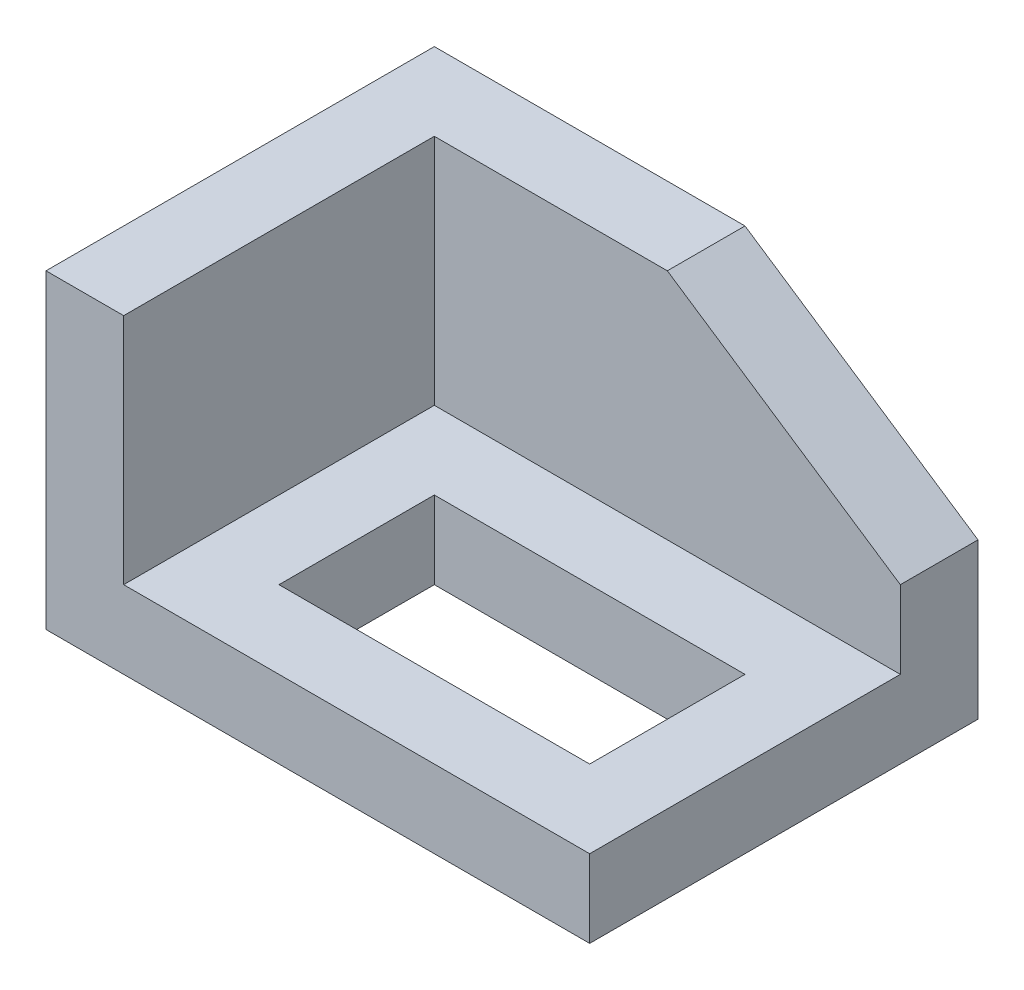
ISO-10303-21;
HEADER;
FILE_DESCRIPTION(('STEP AP214'),'2;1');
FILE_NAME('part.step','',(''),(''),'','','');
FILE_SCHEMA(('AUTOMOTIVE_DESIGN { 1 0 10303 214 1 1 1 1 }'));
ENDSEC;
DATA;
#1=APPLICATION_CONTEXT('core data for automotive mechanical design processes');
#2=APPLICATION_PROTOCOL_DEFINITION('international standard','automotive_design',2000,#1);
#3=PRODUCT_CONTEXT('',#1,'mechanical');
#4=PRODUCT('Part','Part','',(#3));
#5=PRODUCT_RELATED_PRODUCT_CATEGORY('part','',(#4));
#6=PRODUCT_DEFINITION_FORMATION('','',#4);
#7=PRODUCT_DEFINITION_CONTEXT('part definition',#1,'design');
#8=PRODUCT_DEFINITION('design','',#6,#7);
#9=PRODUCT_DEFINITION_SHAPE('','',#8);
#10=(LENGTH_UNIT() NAMED_UNIT(*) SI_UNIT(.MILLI.,.METRE.));
#11=(NAMED_UNIT(*) PLANE_ANGLE_UNIT() SI_UNIT($,.RADIAN.));
#12=(NAMED_UNIT(*) SI_UNIT($,.STERADIAN.) SOLID_ANGLE_UNIT());
#13=UNCERTAINTY_MEASURE_WITH_UNIT(LENGTH_MEASURE(1.E-05),#10,'distance_accuracy_value','');
#14=(GEOMETRIC_REPRESENTATION_CONTEXT(3) GLOBAL_UNCERTAINTY_ASSIGNED_CONTEXT((#13)) GLOBAL_UNIT_ASSIGNED_CONTEXT((#10,
#11,#12)) REPRESENTATION_CONTEXT('',''));
#15=CARTESIAN_POINT('',(0.,0.,0.));
#16=DIRECTION('',(0.,0.,1.));
#17=DIRECTION('',(1.,0.,0.));
#18=AXIS2_PLACEMENT_3D('',#15,#16,#17);
#19=CARTESIAN_POINT('',(0.,0.,10.));
#20=DIRECTION('',(0.,0.,1.));
#21=DIRECTION('',(1.,0.,0.));
#22=AXIS2_PLACEMENT_3D('',#19,#20,#21);
#23=PLANE('',#22);
#24=DIRECTION('',(0.,1.,0.));
#25=VECTOR('',#24,1.);
#26=CARTESIAN_POINT('',(10.,40.,10.));
#27=LINE('',#26,#25);
#28=CARTESIAN_POINT('',(10.,10.,10.));
#29=VERTEX_POINT('',#28);
#30=CARTESIAN_POINT('',(10.,40.,10.));
#31=VERTEX_POINT('',#30);
#32=EDGE_CURVE('E182',#29,#31,#27,.T.);
#33=ORIENTED_EDGE('',*,*,#32,.F.);
#34=DIRECTION('',(-1.,0.,0.));
#35=VECTOR('',#34,1.);
#36=CARTESIAN_POINT('',(10.,10.,10.));
#37=LINE('',#36,#35);
#38=CARTESIAN_POINT('',(70.,10.,10.));
#39=VERTEX_POINT('',#38);
#40=EDGE_CURVE('E167',#39,#29,#37,.T.);
#41=ORIENTED_EDGE('',*,*,#40,.F.);
#42=DIRECTION('',(0.,1.,0.));
#43=VECTOR('',#42,1.);
#44=CARTESIAN_POINT('',(70.,0.,10.));
#45=LINE('',#44,#43);
#46=CARTESIAN_POINT('',(70.,20.,10.));
#47=VERTEX_POINT('',#46);
#48=EDGE_CURVE('E196',#39,#47,#45,.T.);
#49=ORIENTED_EDGE('',*,*,#48,.T.);
#50=DIRECTION('',(-0.832050294337844,0.554700196225229,0.));
#51=VECTOR('',#50,1.);
#52=CARTESIAN_POINT('',(70.,20.,10.));
#53=LINE('',#52,#51);
#54=CARTESIAN_POINT('',(40.,40.,10.));
#55=VERTEX_POINT('',#54);
#56=EDGE_CURVE('E199',#47,#55,#53,.T.);
#57=ORIENTED_EDGE('',*,*,#56,.T.);
#58=DIRECTION('',(-1.,0.,0.));
#59=VECTOR('',#58,1.);
#60=CARTESIAN_POINT('',(0.,40.,10.));
#61=LINE('',#60,#59);
#62=EDGE_CURVE('E201',#55,#31,#61,.T.);
#63=ORIENTED_EDGE('',*,*,#62,.T.);
#64=EDGE_LOOP('',(#33,#41,#49,#57,#63));
#65=FACE_BOUND('',#64,.T.);
#66=ADVANCED_FACE('F44',(#65),#23,.T.);
#67=CARTESIAN_POINT('',(10.,40.,50.));
#68=DIRECTION('',(-1.,0.,0.));
#69=DIRECTION('',(0.,-1.,0.));
#70=AXIS2_PLACEMENT_3D('',#67,#68,#69);
#71=PLANE('',#70);
#72=DIRECTION('',(0.,0.,-1.));
#73=VECTOR('',#72,1.);
#74=CARTESIAN_POINT('',(10.,10.,50.));
#75=LINE('',#74,#73);
#76=CARTESIAN_POINT('',(10.,10.,50.));
#77=VERTEX_POINT('',#76);
#78=EDGE_CURVE('E172',#77,#29,#75,.T.);
#79=ORIENTED_EDGE('',*,*,#78,.T.);
#80=ORIENTED_EDGE('',*,*,#32,.T.);
#81=DIRECTION('',(0.,0.,-1.));
#82=VECTOR('',#81,1.);
#83=CARTESIAN_POINT('',(10.,40.,50.));
#84=LINE('',#83,#82);
#85=CARTESIAN_POINT('',(10.,40.,50.));
#86=VERTEX_POINT('',#85);
#87=EDGE_CURVE('E191',#86,#31,#84,.T.);
#88=ORIENTED_EDGE('',*,*,#87,.F.);
#89=DIRECTION('',(0.,1.,0.));
#90=VECTOR('',#89,1.);
#91=CARTESIAN_POINT('',(10.,40.,50.));
#92=LINE('',#91,#90);
#93=EDGE_CURVE('E190',#77,#86,#92,.T.);
#94=ORIENTED_EDGE('',*,*,#93,.F.);
#95=EDGE_LOOP('',(#79,#80,#88,#94));
#96=FACE_BOUND('',#95,.T.);
#97=ADVANCED_FACE('F253',(#96),#71,.F.);
#98=CARTESIAN_POINT('',(0.,0.,10.));
#99=DIRECTION('',(0.,1.,0.));
#100=DIRECTION('',(0.,0.,1.));
#101=AXIS2_PLACEMENT_3D('',#98,#99,#100);
#102=PLANE('',#101);
#103=DIRECTION('',(-1.,0.,0.));
#104=VECTOR('',#103,1.);
#105=CARTESIAN_POINT('',(20.,0.,20.));
#106=LINE('',#105,#104);
#107=CARTESIAN_POINT('',(60.,0.,20.));
#108=VERTEX_POINT('',#107);
#109=CARTESIAN_POINT('',(20.,0.,20.));
#110=VERTEX_POINT('',#109);
#111=EDGE_CURVE('E142',#108,#110,#106,.T.);
#112=ORIENTED_EDGE('',*,*,#111,.T.);
#113=DIRECTION('',(0.,0.,1.));
#114=VECTOR('',#113,1.);
#115=CARTESIAN_POINT('',(20.,0.,20.));
#116=LINE('',#115,#114);
#117=CARTESIAN_POINT('',(20.,0.,40.));
#118=VERTEX_POINT('',#117);
#119=EDGE_CURVE('E138',#110,#118,#116,.T.);
#120=ORIENTED_EDGE('',*,*,#119,.T.);
#121=DIRECTION('',(1.,0.,0.));
#122=VECTOR('',#121,1.);
#123=CARTESIAN_POINT('',(20.,0.,40.));
#124=LINE('',#123,#122);
#125=CARTESIAN_POINT('',(60.,0.,40.));
#126=VERTEX_POINT('',#125);
#127=EDGE_CURVE('E144',#118,#126,#124,.T.);
#128=ORIENTED_EDGE('',*,*,#127,.T.);
#129=DIRECTION('',(0.,0.,-1.));
#130=VECTOR('',#129,1.);
#131=CARTESIAN_POINT('',(60.,0.,20.));
#132=LINE('',#131,#130);
#133=EDGE_CURVE('E58',#126,#108,#132,.T.);
#134=ORIENTED_EDGE('',*,*,#133,.T.);
#135=EDGE_LOOP('',(#112,#120,#128,#134));
#136=FACE_BOUND('',#135,.T.);
#137=DIRECTION('',(0.,0.,-1.));
#138=VECTOR('',#137,1.);
#139=CARTESIAN_POINT('',(70.,0.,10.));
#140=LINE('',#139,#138);
#141=CARTESIAN_POINT('',(70.,0.,50.));
#142=VERTEX_POINT('',#141);
#143=CARTESIAN_POINT('',(70.,0.,0.));
#144=VERTEX_POINT('',#143);
#145=EDGE_CURVE('E11',#142,#144,#140,.T.);
#146=ORIENTED_EDGE('',*,*,#145,.F.);
#147=DIRECTION('',(1.,0.,0.));
#148=VECTOR('',#147,1.);
#149=CARTESIAN_POINT('',(0.,0.,50.));
#150=LINE('',#149,#148);
#151=CARTESIAN_POINT('',(0.,0.,50.));
#152=VERTEX_POINT('',#151);
#153=EDGE_CURVE('E183',#152,#142,#150,.T.);
#154=ORIENTED_EDGE('',*,*,#153,.F.);
#155=DIRECTION('',(0.,0.,-1.));
#156=VECTOR('',#155,1.);
#157=CARTESIAN_POINT('',(0.,0.,10.));
#158=LINE('',#157,#156);
#159=CARTESIAN_POINT('',(0.,0.,0.));
#160=VERTEX_POINT('',#159);
#161=EDGE_CURVE('E206',#152,#160,#158,.T.);
#162=ORIENTED_EDGE('',*,*,#161,.T.);
#163=DIRECTION('',(1.,0.,0.));
#164=VECTOR('',#163,1.);
#165=CARTESIAN_POINT('',(0.,0.,0.));
#166=LINE('',#165,#164);
#167=EDGE_CURVE('E197',#160,#144,#166,.T.);
#168=ORIENTED_EDGE('',*,*,#167,.T.);
#169=EDGE_LOOP('',(#146,#154,#162,#168));
#170=FACE_BOUND('',#169,.T.);
#171=ADVANCED_FACE('F50',(#136,#170),#102,.F.);
#172=CARTESIAN_POINT('',(70.,0.,10.));
#173=DIRECTION('',(-1.,0.,0.));
#174=DIRECTION('',(0.,0.,1.));
#175=AXIS2_PLACEMENT_3D('',#172,#173,#174);
#176=PLANE('',#175);
#177=DIRECTION('',(0.,1.,0.));
#178=VECTOR('',#177,1.);
#179=CARTESIAN_POINT('',(70.,0.,0.));
#180=LINE('',#179,#178);
#181=CARTESIAN_POINT('',(70.,20.,0.));
#182=VERTEX_POINT('',#181);
#183=EDGE_CURVE('E207',#144,#182,#180,.T.);
#184=ORIENTED_EDGE('',*,*,#183,.T.);
#185=DIRECTION('',(0.,0.,-1.));
#186=VECTOR('',#185,1.);
#187=CARTESIAN_POINT('',(70.,20.,10.));
#188=LINE('',#187,#186);
#189=EDGE_CURVE('E52',#47,#182,#188,.T.);
#190=ORIENTED_EDGE('',*,*,#189,.F.);
#191=ORIENTED_EDGE('',*,*,#48,.F.);
#192=DIRECTION('',(0.,0.,-1.));
#193=VECTOR('',#192,1.);
#194=CARTESIAN_POINT('',(70.,10.,50.));
#195=LINE('',#194,#193);
#196=CARTESIAN_POINT('',(70.,10.,50.));
#197=VERTEX_POINT('',#196);
#198=EDGE_CURVE('E179',#197,#39,#195,.T.);
#199=ORIENTED_EDGE('',*,*,#198,.F.);
#200=DIRECTION('',(0.,1.,0.));
#201=VECTOR('',#200,1.);
#202=CARTESIAN_POINT('',(70.,0.,50.));
#203=LINE('',#202,#201);
#204=EDGE_CURVE('E168',#142,#197,#203,.T.);
#205=ORIENTED_EDGE('',*,*,#204,.F.);
#206=ORIENTED_EDGE('',*,*,#145,.T.);
#207=EDGE_LOOP('',(#184,#190,#191,#199,#205,#206));
#208=FACE_BOUND('',#207,.T.);
#209=ADVANCED_FACE('F258',(#208),#176,.F.);
#210=CARTESIAN_POINT('',(70.,20.,10.));
#211=DIRECTION('',(-0.554700196225229,-0.832050294337844,0.));
#212=DIRECTION('',(0.832050294337844,-0.554700196225229,0.));
#213=AXIS2_PLACEMENT_3D('',#210,#211,#212);
#214=PLANE('',#213);
#215=DIRECTION('',(-0.832050294337844,0.554700196225229,0.));
#216=VECTOR('',#215,1.);
#217=CARTESIAN_POINT('',(70.,20.,0.));
#218=LINE('',#217,#216);
#219=CARTESIAN_POINT('',(40.,40.,0.));
#220=VERTEX_POINT('',#219);
#221=EDGE_CURVE('E211',#182,#220,#218,.T.);
#222=ORIENTED_EDGE('',*,*,#221,.T.);
#223=DIRECTION('',(0.,0.,-1.));
#224=VECTOR('',#223,1.);
#225=CARTESIAN_POINT('',(40.,40.,10.));
#226=LINE('',#225,#224);
#227=EDGE_CURVE('E222',#55,#220,#226,.T.);
#228=ORIENTED_EDGE('',*,*,#227,.F.);
#229=ORIENTED_EDGE('',*,*,#56,.F.);
#230=ORIENTED_EDGE('',*,*,#189,.T.);
#231=EDGE_LOOP('',(#222,#228,#229,#230));
#232=FACE_BOUND('',#231,.T.);
#233=ADVANCED_FACE('F230',(#232),#214,.F.);
#234=CARTESIAN_POINT('',(0.,40.,10.));
#235=DIRECTION('',(0.,-1.,0.));
#236=DIRECTION('',(0.,0.,-1.));
#237=AXIS2_PLACEMENT_3D('',#234,#235,#236);
#238=PLANE('',#237);
#239=DIRECTION('',(-1.,0.,0.));
#240=VECTOR('',#239,1.);
#241=CARTESIAN_POINT('',(0.,40.,0.));
#242=LINE('',#241,#240);
#243=CARTESIAN_POINT('',(0.,40.,0.));
#244=VERTEX_POINT('',#243);
#245=EDGE_CURVE('E213',#220,#244,#242,.T.);
#246=ORIENTED_EDGE('',*,*,#245,.T.);
#247=DIRECTION('',(0.,0.,-1.));
#248=VECTOR('',#247,1.);
#249=CARTESIAN_POINT('',(0.,40.,10.));
#250=LINE('',#249,#248);
#251=CARTESIAN_POINT('',(0.,40.,50.));
#252=VERTEX_POINT('',#251);
#253=EDGE_CURVE('E217',#252,#244,#250,.T.);
#254=ORIENTED_EDGE('',*,*,#253,.F.);
#255=DIRECTION('',(-1.,0.,0.));
#256=VECTOR('',#255,1.);
#257=CARTESIAN_POINT('',(0.,40.,50.));
#258=LINE('',#257,#256);
#259=EDGE_CURVE('E187',#86,#252,#258,.T.);
#260=ORIENTED_EDGE('',*,*,#259,.F.);
#261=ORIENTED_EDGE('',*,*,#87,.T.);
#262=ORIENTED_EDGE('',*,*,#62,.F.);
#263=ORIENTED_EDGE('',*,*,#227,.T.);
#264=EDGE_LOOP('',(#246,#254,#260,#261,#262,#263));
#265=FACE_BOUND('',#264,.T.);
#266=ADVANCED_FACE('F236',(#265),#238,.F.);
#267=CARTESIAN_POINT('',(0.,0.,10.));
#268=DIRECTION('',(1.,0.,0.));
#269=DIRECTION('',(0.,0.,-1.));
#270=AXIS2_PLACEMENT_3D('',#267,#268,#269);
#271=PLANE('',#270);
#272=DIRECTION('',(0.,-1.,0.));
#273=VECTOR('',#272,1.);
#274=CARTESIAN_POINT('',(0.,0.,0.));
#275=LINE('',#274,#273);
#276=EDGE_CURVE('E203',#244,#160,#275,.T.);
#277=ORIENTED_EDGE('',*,*,#276,.T.);
#278=ORIENTED_EDGE('',*,*,#161,.F.);
#279=DIRECTION('',(0.,-1.,0.));
#280=VECTOR('',#279,1.);
#281=CARTESIAN_POINT('',(0.,40.,50.));
#282=LINE('',#281,#280);
#283=EDGE_CURVE('E185',#252,#152,#282,.T.);
#284=ORIENTED_EDGE('',*,*,#283,.F.);
#285=ORIENTED_EDGE('',*,*,#253,.T.);
#286=EDGE_LOOP('',(#277,#278,#284,#285));
#287=FACE_BOUND('',#286,.T.);
#288=ADVANCED_FACE('F245',(#287),#271,.F.);
#289=CARTESIAN_POINT('',(0.,0.,0.));
#290=DIRECTION('',(0.,0.,1.));
#291=DIRECTION('',(1.,0.,0.));
#292=AXIS2_PLACEMENT_3D('',#289,#290,#291);
#293=PLANE('',#292);
#294=ORIENTED_EDGE('',*,*,#167,.F.);
#295=ORIENTED_EDGE('',*,*,#276,.F.);
#296=ORIENTED_EDGE('',*,*,#245,.F.);
#297=ORIENTED_EDGE('',*,*,#221,.F.);
#298=ORIENTED_EDGE('',*,*,#183,.F.);
#299=EDGE_LOOP('',(#294,#295,#296,#297,#298));
#300=FACE_BOUND('',#299,.T.);
#301=ADVANCED_FACE('F232',(#300),#293,.F.);
#302=CARTESIAN_POINT('',(0.,0.,50.));
#303=DIRECTION('',(0.,0.,1.));
#304=DIRECTION('',(1.,0.,0.));
#305=AXIS2_PLACEMENT_3D('',#302,#303,#304);
#306=PLANE('',#305);
#307=ORIENTED_EDGE('',*,*,#283,.T.);
#308=ORIENTED_EDGE('',*,*,#153,.T.);
#309=ORIENTED_EDGE('',*,*,#204,.T.);
#310=DIRECTION('',(-1.,0.,0.));
#311=VECTOR('',#310,1.);
#312=CARTESIAN_POINT('',(10.,10.,50.));
#313=LINE('',#312,#311);
#314=EDGE_CURVE('E171',#197,#77,#313,.T.);
#315=ORIENTED_EDGE('',*,*,#314,.T.);
#316=ORIENTED_EDGE('',*,*,#93,.T.);
#317=ORIENTED_EDGE('',*,*,#259,.T.);
#318=EDGE_LOOP('',(#307,#308,#309,#315,#316,#317));
#319=FACE_BOUND('',#318,.T.);
#320=ADVANCED_FACE('F248',(#319),#306,.T.);
#321=CARTESIAN_POINT('',(10.,10.,50.));
#322=DIRECTION('',(0.,-1.,0.));
#323=DIRECTION('',(0.,0.,-1.));
#324=AXIS2_PLACEMENT_3D('',#321,#322,#323);
#325=PLANE('',#324);
#326=DIRECTION('',(1.,0.,0.));
#327=VECTOR('',#326,1.);
#328=CARTESIAN_POINT('',(20.,10.,40.));
#329=LINE('',#328,#327);
#330=CARTESIAN_POINT('',(20.,10.,40.));
#331=VERTEX_POINT('',#330);
#332=CARTESIAN_POINT('',(60.,10.,40.));
#333=VERTEX_POINT('',#332);
#334=EDGE_CURVE('E159',#331,#333,#329,.T.);
#335=ORIENTED_EDGE('',*,*,#334,.F.);
#336=DIRECTION('',(0.,0.,1.));
#337=VECTOR('',#336,1.);
#338=CARTESIAN_POINT('',(20.,10.,20.));
#339=LINE('',#338,#337);
#340=CARTESIAN_POINT('',(20.,10.,20.));
#341=VERTEX_POINT('',#340);
#342=EDGE_CURVE('E66',#341,#331,#339,.T.);
#343=ORIENTED_EDGE('',*,*,#342,.F.);
#344=DIRECTION('',(-1.,0.,0.));
#345=VECTOR('',#344,1.);
#346=CARTESIAN_POINT('',(20.,10.,20.));
#347=LINE('',#346,#345);
#348=CARTESIAN_POINT('',(60.,10.,20.));
#349=VERTEX_POINT('',#348);
#350=EDGE_CURVE('E151',#349,#341,#347,.T.);
#351=ORIENTED_EDGE('',*,*,#350,.F.);
#352=DIRECTION('',(0.,0.,-1.));
#353=VECTOR('',#352,1.);
#354=CARTESIAN_POINT('',(60.,10.,20.));
#355=LINE('',#354,#353);
#356=EDGE_CURVE('E152',#333,#349,#355,.T.);
#357=ORIENTED_EDGE('',*,*,#356,.F.);
#358=EDGE_LOOP('',(#335,#343,#351,#357));
#359=FACE_BOUND('',#358,.T.);
#360=ORIENTED_EDGE('',*,*,#40,.T.);
#361=ORIENTED_EDGE('',*,*,#78,.F.);
#362=ORIENTED_EDGE('',*,*,#314,.F.);
#363=ORIENTED_EDGE('',*,*,#198,.T.);
#364=EDGE_LOOP('',(#360,#361,#362,#363));
#365=FACE_BOUND('',#364,.T.);
#366=ADVANCED_FACE('F259',(#359,#365),#325,.F.);
#367=CARTESIAN_POINT('',(20.,0.,20.));
#368=DIRECTION('',(-1.,0.,0.));
#369=DIRECTION('',(0.,0.,1.));
#370=AXIS2_PLACEMENT_3D('',#367,#368,#369);
#371=PLANE('',#370);
#372=ORIENTED_EDGE('',*,*,#342,.T.);
#373=DIRECTION('',(0.,1.,0.));
#374=VECTOR('',#373,1.);
#375=CARTESIAN_POINT('',(20.,0.,40.));
#376=LINE('',#375,#374);
#377=EDGE_CURVE('E131',#118,#331,#376,.T.);
#378=ORIENTED_EDGE('',*,*,#377,.F.);
#379=ORIENTED_EDGE('',*,*,#119,.F.);
#380=DIRECTION('',(0.,1.,0.));
#381=VECTOR('',#380,1.);
#382=CARTESIAN_POINT('',(20.,0.,20.));
#383=LINE('',#382,#381);
#384=EDGE_CURVE('E163',#110,#341,#383,.T.);
#385=ORIENTED_EDGE('',*,*,#384,.T.);
#386=EDGE_LOOP('',(#372,#378,#379,#385));
#387=FACE_BOUND('',#386,.T.);
#388=ADVANCED_FACE('F133',(#387),#371,.F.);
#389=CARTESIAN_POINT('',(20.,0.,20.));
#390=DIRECTION('',(0.,0.,-1.));
#391=DIRECTION('',(-1.,0.,0.));
#392=AXIS2_PLACEMENT_3D('',#389,#390,#391);
#393=PLANE('',#392);
#394=ORIENTED_EDGE('',*,*,#350,.T.);
#395=ORIENTED_EDGE('',*,*,#384,.F.);
#396=ORIENTED_EDGE('',*,*,#111,.F.);
#397=DIRECTION('',(0.,1.,0.));
#398=VECTOR('',#397,1.);
#399=CARTESIAN_POINT('',(60.,0.,20.));
#400=LINE('',#399,#398);
#401=EDGE_CURVE('E170',#108,#349,#400,.T.);
#402=ORIENTED_EDGE('',*,*,#401,.T.);
#403=EDGE_LOOP('',(#394,#395,#396,#402));
#404=FACE_BOUND('',#403,.T.);
#405=ADVANCED_FACE('F270',(#404),#393,.F.);
#406=CARTESIAN_POINT('',(60.,0.,20.));
#407=DIRECTION('',(1.,0.,0.));
#408=DIRECTION('',(0.,0.,-1.));
#409=AXIS2_PLACEMENT_3D('',#406,#407,#408);
#410=PLANE('',#409);
#411=ORIENTED_EDGE('',*,*,#356,.T.);
#412=ORIENTED_EDGE('',*,*,#401,.F.);
#413=ORIENTED_EDGE('',*,*,#133,.F.);
#414=DIRECTION('',(0.,1.,0.));
#415=VECTOR('',#414,1.);
#416=CARTESIAN_POINT('',(60.,0.,40.));
#417=LINE('',#416,#415);
#418=EDGE_CURVE('E143',#126,#333,#417,.T.);
#419=ORIENTED_EDGE('',*,*,#418,.T.);
#420=EDGE_LOOP('',(#411,#412,#413,#419));
#421=FACE_BOUND('',#420,.T.);
#422=ADVANCED_FACE('F323',(#421),#410,.F.);
#423=CARTESIAN_POINT('',(20.,0.,40.));
#424=DIRECTION('',(0.,0.,1.));
#425=DIRECTION('',(1.,0.,0.));
#426=AXIS2_PLACEMENT_3D('',#423,#424,#425);
#427=PLANE('',#426);
#428=ORIENTED_EDGE('',*,*,#334,.T.);
#429=ORIENTED_EDGE('',*,*,#418,.F.);
#430=ORIENTED_EDGE('',*,*,#127,.F.);
#431=ORIENTED_EDGE('',*,*,#377,.T.);
#432=EDGE_LOOP('',(#428,#429,#430,#431));
#433=FACE_BOUND('',#432,.T.);
#434=ADVANCED_FACE('F148',(#433),#427,.F.);
#435=CLOSED_SHELL('',(#66,#97,#171,#209,#233,#266,#288,#301,#320,#366,#388,#405,#422,#434));
#436=MANIFOLD_SOLID_BREP('B2',#435);
#437=ADVANCED_BREP_SHAPE_REPRESENTATION('',(#18,#436),#14);
#438=SHAPE_DEFINITION_REPRESENTATION(#9,#437);
ENDSEC;
END-ISO-10303-21;
